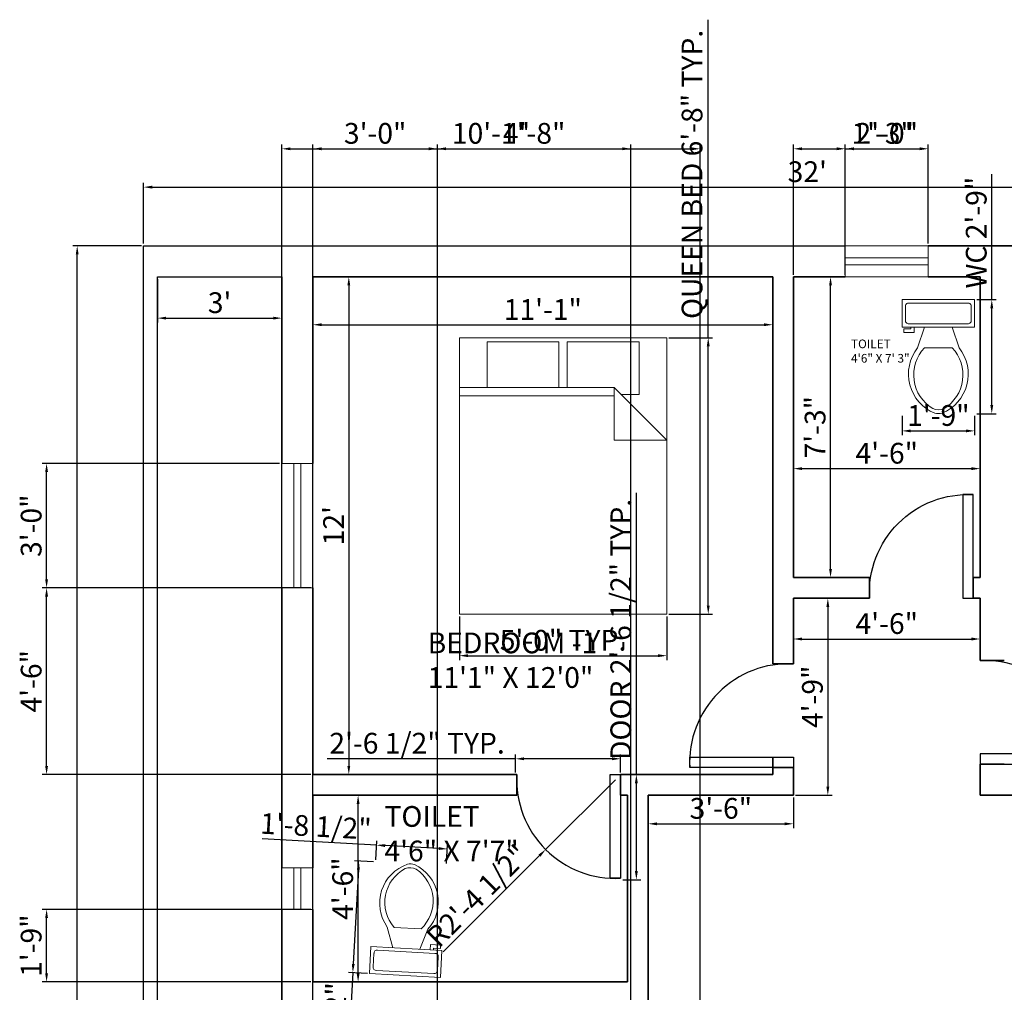
# Model space of a CAD drawing. Units: inches. Extents: x 2117 to 2588, y 1610 to 2201.
# Tile 3 of 4: x 2122 to 2407, y 1920 to 2201. Entities that reach past the tile are written whole.
import ezdxf

# ---------------------------------------------------------------- set-up
doc = ezdxf.new("R2010")
doc.units = ezdxf.units.IN
for name, color, linetype, lineweight in [('A-ANNO-DIMS', 2, 'Continuous', 18), ('A-AREA-IDEN', 7, 'Continuous', 25), ('A-DOOR', 4, 'Continuous', 25), ('A-FLOR-FIXT', 9, 'Continuous', 18), ('A-FURN', 8, 'Continuous', 18), ('A-WALL', 7, 'Continuous', 35), ('C-PROP', 7, 'Continuous', 30), ('WINDOW', 150, 'Continuous', 18)]:
    doc.layers.add(name, color=color, linetype=linetype, lineweight=lineweight)
doc.styles.get("Standard").update_dxf_attribs({"font": 'arial.ttf'})
doc.dimstyles.new('ISO-25', dxfattribs={"dimtxt": 6, "dimasz": 2.5, "dimexe": 1.25, "dimexo": 0.625, "dimtad": 1, "dimlunit": 3, "dimtxsty": 'Standard', "dimcen": 2.5, "dimadec": 0, "dimazin": 0, "dimtfac": 1, "dimtmove": 0, "dimatfit": 3, "dimfxl": 1, "dimarcsym": 0})

# ---------------------------------------------------------------- blocks, each defined once
blk = doc.blocks.new('*D3')
at = {"layer": 'A-ANNO-DIMS', "color": 0, "lineweight": -2, "transparency": 16777216}
for p, q in [((2346.08, 2126.4), (2346.08, 2070.29)), ((2400.08, 2126.4), (2400.08, 2070.29)), ((2348.58, 2071.54), (2397.58, 2071.54))]:
    blk.add_line(p, q, dxfattribs=at)
at = {"layer": 'A-ANNO-DIMS', "color": 0, "transparency": 16777216}
for points in [[(2348.58, 2071.95), (2348.58, 2071.12), (2346.08, 2071.54)], [(2397.58, 2071.95), (2397.58, 2071.12), (2400.08, 2071.54)]]:
    blk.add_solid(points, dxfattribs=at)
at = {"layer": 'Defpoints', "color": 0, "transparency": 16777216}
for p in [(2346.08, 2127.03), (2400.08, 2127.03), (2400.08, 2071.54)]:
    blk.add_point(p, dxfattribs=at)
at = {"layer": 'A-ANNO-DIMS', "color": 0, "transparency": 16777216, "insert": (2373.08, 2075.22), "char_height": 6, "attachment_point": 5}
blk.add_mtext('4\'-6"', dxfattribs=at)
blk = doc.blocks.new('*D4')
at = {"layer": 'A-ANNO-DIMS', "color": 0, "lineweight": -2, "transparency": 16777216}
for p, q in [((2207.7, 2127.03), (2218.7, 2127.03)), ((2217.45, 2124.53), (2217.45, 1985.53)), ((2207.7, 1983.03), (2218.7, 1983.03))]:
    blk.add_line(p, q, dxfattribs=at)
at = {"layer": 'A-ANNO-DIMS', "color": 0, "transparency": 16777216}
for points in [[(2217.04, 2124.53), (2217.87, 2124.53), (2217.45, 2127.03)], [(2217.04, 1985.53), (2217.87, 1985.53), (2217.45, 1983.03)]]:
    blk.add_solid(points, dxfattribs=at)
at = {"layer": 'Defpoints', "color": 0, "transparency": 16777216}
for p in [(2207.08, 2127.03), (2207.08, 1983.03), (2217.45, 1983.03)]:
    blk.add_point(p, dxfattribs=at)
at = {"layer": 'A-ANNO-DIMS', "color": 0, "transparency": 16777216, "insert": (2213.82, 2055.03), "char_height": 6, "attachment_point": 5, "rotation": 90}
blk.add_mtext("12'", dxfattribs=at)
blk = doc.blocks.new('*D7')
at = {"layer": 'A-ANNO-DIMS', "color": 0, "lineweight": -2, "transparency": 16777216}
for p, q in [((2207.7, 1977.03), (2221.4, 1977.03)), ((2220.15, 1925.53), (2220.15, 1974.53)), ((2207.7, 1923.03), (2221.4, 1923.03))]:
    blk.add_line(p, q, dxfattribs=at)
at = {"layer": 'A-ANNO-DIMS', "color": 0, "transparency": 16777216}
for points in [[(2219.73, 1974.53), (2220.56, 1974.53), (2220.15, 1977.03)], [(2219.73, 1925.53), (2220.56, 1925.53), (2220.15, 1923.03)]]:
    blk.add_solid(points, dxfattribs=at)
at = {"layer": 'Defpoints', "color": 0, "transparency": 16777216}
for p in [(2207.08, 1977.03), (2220.15, 1977.03), (2207.08, 1923.03)]:
    blk.add_point(p, dxfattribs=at)
at = {"layer": 'A-ANNO-DIMS', "color": 0, "transparency": 16777216, "insert": (2216.46, 1950.03), "char_height": 6, "attachment_point": 5, "rotation": 90}
blk.add_mtext('4\'-6"', dxfattribs=at)
blk = doc.blocks.new('*D9')
at = {"layer": 'A-ANNO-DIMS', "color": 0, "lineweight": -2, "transparency": 16777216}
for p, q in [((2162.08, 2126.4), (2162.08, 2113.83)), ((2198.08, 2126.4), (2198.08, 2113.83)), ((2164.58, 2115.08), (2195.58, 2115.08))]:
    blk.add_line(p, q, dxfattribs=at)
at = {"layer": 'A-ANNO-DIMS', "color": 0, "transparency": 16777216}
for points in [[(2164.58, 2115.5), (2164.58, 2114.67), (2162.08, 2115.08)], [(2195.58, 2115.5), (2195.58, 2114.67), (2198.08, 2115.08)]]:
    blk.add_solid(points, dxfattribs=at)
at = {"layer": 'Defpoints', "color": 0, "transparency": 16777216}
for p in [(2162.08, 2127.03), (2198.08, 2127.03), (2198.08, 2115.08)]:
    blk.add_point(p, dxfattribs=at)
at = {"layer": 'A-ANNO-DIMS', "color": 0, "transparency": 16777216, "insert": (2180.08, 2118.78), "char_height": 6, "attachment_point": 5}
blk.add_mtext("3'", dxfattribs=at)
blk = doc.blocks.new('*D10')
at = {"layer": 'A-ANNO-DIMS', "color": 0, "lineweight": -2, "transparency": 16777216}
for p, q in [((2207.08, 2126.4), (2207.08, 2111.92)), ((2340.08, 2126.4), (2340.08, 2111.92)), ((2209.58, 2113.17), (2337.58, 2113.17))]:
    blk.add_line(p, q, dxfattribs=at)
at = {"layer": 'A-ANNO-DIMS', "color": 0, "transparency": 16777216}
for points in [[(2209.58, 2113.59), (2209.58, 2112.76), (2207.08, 2113.17)], [(2337.58, 2113.59), (2337.58, 2112.76), (2340.08, 2113.17)]]:
    blk.add_solid(points, dxfattribs=at)
at = {"layer": 'Defpoints', "color": 0, "transparency": 16777216}
for p in [(2207.08, 2127.03), (2340.08, 2127.03), (2340.08, 2113.17)]:
    blk.add_point(p, dxfattribs=at)
at = {"layer": 'A-ANNO-DIMS', "color": 0, "transparency": 16777216, "insert": (2273.58, 2116.81), "char_height": 6, "attachment_point": 5}
blk.add_mtext('11\'-1"', dxfattribs=at)
blk = doc.blocks.new('*D11')
at = {"layer": 'A-ANNO-DIMS', "color": 0, "lineweight": -2, "transparency": 16777216}
for p, q in [((2346.7, 2127.03), (2358.06, 2127.03)), ((2356.81, 2042.53), (2356.81, 2124.53)), ((2346.7, 2040.03), (2358.06, 2040.03))]:
    blk.add_line(p, q, dxfattribs=at)
at = {"layer": 'A-ANNO-DIMS', "color": 0, "transparency": 16777216}
for points in [[(2356.39, 2124.53), (2357.22, 2124.53), (2356.81, 2127.03)], [(2356.39, 2042.53), (2357.22, 2042.53), (2356.81, 2040.03)]]:
    blk.add_solid(points, dxfattribs=at)
at = {"layer": 'Defpoints', "color": 0, "transparency": 16777216}
for p in [(2346.08, 2127.03), (2356.81, 2127.03), (2346.08, 2040.03)]:
    blk.add_point(p, dxfattribs=at)
at = {"layer": 'A-ANNO-DIMS', "color": 0, "transparency": 16777216, "insert": (2353.12, 2083.53), "char_height": 6, "attachment_point": 5, "rotation": 90}
blk.add_mtext('7\'-3"', dxfattribs=at)
blk = doc.blocks.new('*D12')
at = {"layer": 'A-ANNO-DIMS', "color": 0, "lineweight": -2, "transparency": 16777216}
for p, q in [((2346.7, 2034.03), (2357.28, 2034.03)), ((2356.03, 2031.53), (2356.03, 1979.53)), ((2346.7, 1977.03), (2357.28, 1977.03))]:
    blk.add_line(p, q, dxfattribs=at)
at = {"layer": 'A-ANNO-DIMS', "color": 0, "transparency": 16777216}
for points in [[(2355.61, 2031.53), (2356.44, 2031.53), (2356.03, 2034.03)], [(2355.61, 1979.53), (2356.44, 1979.53), (2356.03, 1977.03)]]:
    blk.add_solid(points, dxfattribs=at)
at = {"layer": 'Defpoints', "color": 0, "transparency": 16777216}
for p in [(2346.08, 2034.03), (2346.08, 1977.03), (2356.03, 1977.03)]:
    blk.add_point(p, dxfattribs=at)
at = {"layer": 'A-ANNO-DIMS', "color": 0, "transparency": 16777216, "insert": (2352.34, 2005.53), "char_height": 6, "attachment_point": 5, "rotation": 90}
blk.add_mtext('4\'-9"', dxfattribs=at)
blk = doc.blocks.new('*D13')
at = {"layer": 'A-ANNO-DIMS', "color": 0, "lineweight": -2, "transparency": 16777216}
for p, q in [((2346.08, 2033.4), (2346.08, 2021)), ((2400.08, 2033.4), (2400.08, 2021)), ((2348.58, 2022.25), (2397.58, 2022.25))]:
    blk.add_line(p, q, dxfattribs=at)
at = {"layer": 'A-ANNO-DIMS', "color": 0, "transparency": 16777216}
for points in [[(2348.58, 2022.67), (2348.58, 2021.83), (2346.08, 2022.25)], [(2397.58, 2022.67), (2397.58, 2021.83), (2400.08, 2022.25)]]:
    blk.add_solid(points, dxfattribs=at)
at = {"layer": 'Defpoints', "color": 0, "transparency": 16777216}
for p in [(2346.08, 2034.03), (2400.08, 2034.03), (2400.08, 2022.25)]:
    blk.add_point(p, dxfattribs=at)
at = {"layer": 'A-ANNO-DIMS', "color": 0, "transparency": 16777216, "insert": (2373.08, 2025.94), "char_height": 6, "attachment_point": 5}
blk.add_mtext('4\'-6"', dxfattribs=at)
blk = doc.blocks.new('*D14')
at = {"layer": 'A-ANNO-DIMS', "color": 0, "lineweight": -2, "transparency": 16777216}
for p, q in [((2304.08, 1976.4), (2304.08, 1967.53)), ((2346.08, 1976.4), (2346.08, 1967.53)), ((2306.58, 1968.78), (2343.58, 1968.78))]:
    blk.add_line(p, q, dxfattribs=at)
at = {"layer": 'A-ANNO-DIMS', "color": 0, "transparency": 16777216}
for points in [[(2306.58, 1969.19), (2306.58, 1968.36), (2304.08, 1968.78)], [(2343.58, 1969.19), (2343.58, 1968.36), (2346.08, 1968.78)]]:
    blk.add_solid(points, dxfattribs=at)
at = {"layer": 'Defpoints', "color": 0, "transparency": 16777216}
for p in [(2304.08, 1977.03), (2346.08, 1977.03), (2346.08, 1968.78)]:
    blk.add_point(p, dxfattribs=at)
at = {"layer": 'A-ANNO-DIMS', "color": 0, "transparency": 16777216, "insert": (2325.08, 1972.47), "char_height": 6, "attachment_point": 5}
blk.add_mtext('3\'-6"', dxfattribs=at)
blk = doc.blocks.new('Bed - Queen')
for p, q in [((0, -80.00003), (0, 0)), ((0, 0), (59.99999, 0)), ((59.99999, 0), (59.99999, -80.00003)), ((7.99999, -1.2), (28.79998, -1.2)), ((7.99999, -14.4), (7.99999, -1.2)), ((28.79998, -1.2), (28.79998, -14.4)), ((31.19999, -1.2), (51.99999, -1.2)), ((31.19999, -14.4), (31.19999, -1.2)), ((51.99999, -1.2), (51.99999, -16.4)), ((0, -14.4), (44.8, -14.4)), ((44.8, -16.8), (0, -16.8)), ((59.99999, -29.6), (44.8, -14.4)), ((44.8, -14.4), (44.8, -29.6)), ((51.99999, -16.4), (46.79936, -16.4)), ((44.8, -29.6), (59.99999, -29.6)), ((59.99999, -80.00003), (0, -80.00003))]:
    blk.add_line(p, q)
blk = doc.blocks.new('Toilet - top')
for p, q in [((9.5, -6), (9.5, -2)), ((-10, -8.5), (-8, -8.5)), ((-10, -9.5), (-10, -8.5)), ((-8, -8.5), (-8, -8)), ((-7, -8), (-7, -9.5)), ((-4, -8), (-6, -14)), ((4, -8), (6, -14)), ((-7, -9.5), (-10, -9.5)), ((4, -14), (-4, -14))]:
    blk.add_line(p, q)
blk.add_lwpolyline([(10.5, -8), (10.5, 0), (-10.5, 0), (-10.5, -8)], close=True)
for points in [[(-9.5, -2), (-9.5, -6)], [(8.5, -1), (-8.5, -1)], [(-8.5, -7), (8.5, -7)]]:
    blk.add_lwpolyline(points)
for centre, radius, start, end in [((-8.62, -1.88), 0.884, 81.8699, 188.1301), ((8.62, -1.88), 0.884, 351.8699, 98.1301), ((-8.62, -6.12), 0.884, 171.8699, 278.1301), ((8.62, -6.12), 0.884, 261.8699, 8.1301), ((3.52, -21.58), 12.17, 141.4691, 247.9714), ((4.2, -21.82), 11.33, 136.3677, 238.9468), ((-3.52, -21.58), 12.17, 292.0284, 38.5307), ((-4.2, -21.82), 11.33, 301.053, 43.6321), ((0, -27.88), 4, 245.7318, 294.2682), ((0, -29), 4, 254.8605, 285.1395)]:
    blk.add_arc(centre, radius, start, end)
blk = doc.blocks.new('*D30')
at = {"layer": 'A-ANNO-DIMS', "color": 0, "lineweight": -2, "transparency": 16777216}
for p, q in [((2158.08, 2136.65), (2158.08, 2154.24)), ((2542.08, 2136.65), (2542.08, 2154.24)), ((2160.58, 2152.99), (2539.58, 2152.99))]:
    blk.add_line(p, q, dxfattribs=at)
at = {"layer": 'A-ANNO-DIMS', "color": 0, "transparency": 16777216}
for points in [[(2160.58, 2153.4), (2160.58, 2152.57), (2158.08, 2152.99)], [(2539.58, 2153.4), (2539.58, 2152.57), (2542.08, 2152.99)]]:
    blk.add_solid(points, dxfattribs=at)
at = {"layer": 'Defpoints', "color": 0, "transparency": 16777216}
for p in [(2542.08, 2152.99), (2158.08, 2136.03), (2542.08, 2136.03)]:
    blk.add_point(p, dxfattribs=at)
at = {"layer": 'A-ANNO-DIMS', "color": 0, "transparency": 16777216, "insert": (2350.08, 2156.68), "char_height": 6, "attachment_point": 5}
blk.add_mtext("32'", dxfattribs=at)
blk = doc.blocks.new('*D33')
at = {"layer": 'A-ANNO-DIMS', "color": 0, "lineweight": -2, "transparency": 16777216}
for p, q in [((2157.45, 2136.03), (2137.63, 2136.03)), ((2138.88, 1658.53), (2138.88, 2133.53)), ((2157.45, 1656.03), (2137.63, 1656.03))]:
    blk.add_line(p, q, dxfattribs=at)
at = {"layer": 'A-ANNO-DIMS', "color": 0, "transparency": 16777216}
for points in [[(2138.47, 2133.53), (2139.3, 2133.53), (2138.88, 2136.03)], [(2138.47, 1658.53), (2139.3, 1658.53), (2138.88, 1656.03)]]:
    blk.add_solid(points, dxfattribs=at)
at = {"layer": 'Defpoints', "color": 0, "transparency": 16777216}
for p in [(2138.88, 2136.03), (2158.08, 2136.03), (2158.08, 1656.03)]:
    blk.add_point(p, dxfattribs=at)
at = {"layer": 'A-ANNO-DIMS', "color": 0, "transparency": 16777216, "insert": (2135.2, 1896.03), "char_height": 6, "attachment_point": 5, "rotation": 90}
blk.add_mtext("40'", dxfattribs=at)
blk = doc.blocks.new('WIN-12IN-9IN-WALL')
for p, q in [((9, 12), (0, 12)), ((0, 0), (0, 12)), ((3.5, 0), (3.5, 12)), ((5.5, 0), (5.5, 12)), ((9, 0), (9, 12)), ((9, 0), (0, 0))]:
    blk.add_line(p, q)
blk = doc.blocks.new('DOOR-SWING-30IN')
blk.add_lwpolyline([(30.04, 0), (0.04, 0), (0.04, 3), (30.04, 3)], close=True)
blk.add_arc((28.54, 1.5), 28.54, 86.9872, 183.0128)
blk = doc.blocks.new('*D41')
at = {"layer": 'A-ANNO-DIMS', "color": 0, "lineweight": -2, "transparency": 16777216}
for p, q in [((2300.64, 1983.03), (2300.64, 2064.51)), ((2296.7, 1983.03), (2301.89, 1983.03)), ((2300.64, 1955.1), (2300.64, 1980.53)), ((2296.7, 1952.6), (2301.89, 1952.6))]:
    blk.add_line(p, q, dxfattribs=at)
at = {"layer": 'A-ANNO-DIMS', "color": 0, "transparency": 16777216}
for points in [[(2300.22, 1980.53), (2301.06, 1980.53), (2300.64, 1983.03)], [(2300.22, 1955.1), (2301.06, 1955.1), (2300.64, 1952.6)]]:
    blk.add_solid(points, dxfattribs=at)
at = {"layer": 'Defpoints', "color": 0, "transparency": 16777216}
for p in [(2296.08, 1983.03), (2300.64, 1983.03), (2296.08, 1952.6)]:
    blk.add_point(p, dxfattribs=at)
at = {"layer": 'A-ANNO-DIMS', "color": 0, "transparency": 16777216, "insert": (2296.91, 2025.02), "char_height": 6, "attachment_point": 5, "rotation": 90}
blk.add_mtext('DOOR 2\'-6 1/2" TYP.', dxfattribs=at)
blk = doc.blocks.new('*D42')
at = {"layer": 'A-ANNO-DIMS', "color": 0, "lineweight": -2, "transparency": 16777216}
for p, q in [((2265.65, 1983.65), (2265.65, 1988.84)), ((2296.08, 1983.65), (2296.08, 1988.84)), ((2265.65, 1987.59), (2211.24, 1987.59)), ((2293.58, 1987.59), (2268.15, 1987.59))]:
    blk.add_line(p, q, dxfattribs=at)
at = {"layer": 'A-ANNO-DIMS', "color": 0, "transparency": 16777216}
for points in [[(2268.15, 1988.01), (2268.15, 1987.18), (2265.65, 1987.59)], [(2293.58, 1988.01), (2293.58, 1987.18), (2296.08, 1987.59)]]:
    blk.add_solid(points, dxfattribs=at)
at = {"layer": 'Defpoints', "color": 0, "transparency": 16777216}
for p in [(2265.65, 1987.59), (2265.65, 1983.03), (2296.08, 1983.03)]:
    blk.add_point(p, dxfattribs=at)
at = {"layer": 'A-ANNO-DIMS', "color": 0, "transparency": 16777216, "insert": (2237.2, 1991.32), "char_height": 6, "attachment_point": 5}
blk.add_mtext('2\'-6 1/2" TYP.', dxfattribs=at)
blk = doc.blocks.new('*D43')
at = {"layer": 'A-ANNO-DIMS', "color": 0, "lineweight": -2, "transparency": 16777216}
for p, q in [((2321.43, 2109.42), (2321.43, 2201.43)), ((2310.06, 2109.42), (2322.68, 2109.42)), ((2321.43, 2031.92), (2321.43, 2106.92)), ((2310.06, 2029.42), (2322.68, 2029.42))]:
    blk.add_line(p, q, dxfattribs=at)
at = {"layer": 'A-ANNO-DIMS', "color": 0, "transparency": 16777216}
for points in [[(2321.01, 2106.92), (2321.85, 2106.92), (2321.43, 2109.42)], [(2321.01, 2031.92), (2321.85, 2031.92), (2321.43, 2029.42)]]:
    blk.add_solid(points, dxfattribs=at)
at = {"layer": 'Defpoints', "color": 0, "transparency": 16777216}
for p in [(2309.43, 2109.42), (2321.43, 2109.42), (2309.43, 2029.42)]:
    blk.add_point(p, dxfattribs=at)
at = {"layer": 'A-ANNO-DIMS', "color": 0, "transparency": 16777216, "insert": (2317.52, 2156.68), "char_height": 6, "attachment_point": 5, "rotation": 90}
blk.add_mtext('QUEEN BED 6\'-8" TYP.', dxfattribs=at)
blk = doc.blocks.new('*D44')
at = {"layer": 'A-ANNO-DIMS', "color": 0, "lineweight": -2, "transparency": 16777216}
for p, q in [((2249.43, 2028.8), (2249.43, 2016.17)), ((2309.43, 2028.8), (2309.43, 2016.17)), ((2251.93, 2017.42), (2306.93, 2017.42))]:
    blk.add_line(p, q, dxfattribs=at)
at = {"layer": 'A-ANNO-DIMS', "color": 0, "transparency": 16777216}
for points in [[(2251.93, 2017.84), (2251.93, 2017.01), (2249.43, 2017.42)], [(2306.93, 2017.84), (2306.93, 2017.01), (2309.43, 2017.42)]]:
    blk.add_solid(points, dxfattribs=at)
at = {"layer": 'Defpoints', "color": 0, "transparency": 16777216}
for p in [(2249.43, 2029.42), (2309.43, 2029.42), (2309.43, 2017.42)]:
    blk.add_point(p, dxfattribs=at)
at = {"layer": 'A-ANNO-DIMS', "color": 0, "transparency": 16777216, "insert": (2279.43, 2021.11), "char_height": 6, "attachment_point": 5}
blk.add_mtext('5\'-0" TYP.', dxfattribs=at)
blk = doc.blocks.new('*D45')
at = {"layer": 'A-ANNO-DIMS', "color": 0, "lineweight": -2, "transparency": 16777216}
for p, q in [((2224.57, 1957.8), (2219.1, 1958.1)), ((2220.21, 1955.54), (2218.73, 1928.23)), ((2218.6, 1925.73), (2215.87, 1875.58)), ((2222.82, 1925.5), (2217.35, 1925.8))]:
    blk.add_line(p, q, dxfattribs=at)
at = {"layer": 'A-ANNO-DIMS', "color": 0, "transparency": 16777216}
for points in [[(2219.8, 1955.56), (2220.63, 1955.51), (2220.35, 1958.03)], [(2218.32, 1928.25), (2219.15, 1928.2), (2218.6, 1925.73)]]:
    blk.add_solid(points, dxfattribs=at)
at = {"layer": 'Defpoints', "color": 0, "transparency": 16777216}
for p in [(2225.19, 1957.77), (2218.6, 1925.73), (2223.44, 1925.47)]:
    blk.add_point(p, dxfattribs=at)
at = {"layer": 'A-ANNO-DIMS', "color": 0, "transparency": 16777216, "insert": (2213.45, 1899.61), "char_height": 6, "attachment_point": 5, "rotation": 86.894}
blk.add_mtext('WC 2\'-8 1/2"', dxfattribs=at)
blk = doc.blocks.new('*D46')
at = {"layer": 'A-ANNO-DIMS', "color": 0, "lineweight": -2, "transparency": 16777216}
for p, q in [((2225.46, 1962.61), (2192.39, 1964.41)), ((2225.23, 1958.39), (2225.52, 1963.86)), ((2243.49, 1961.64), (2227.95, 1962.48)), ((2245.76, 1957.28), (2246.05, 1962.75))]:
    blk.add_line(p, q, dxfattribs=at)
at = {"layer": 'A-ANNO-DIMS', "color": 0, "transparency": 16777216}
for points in [[(2227.98, 1962.9), (2227.93, 1962.06), (2225.46, 1962.61)], [(2243.51, 1962.05), (2243.47, 1961.22), (2245.98, 1961.5)]]:
    blk.add_solid(points, dxfattribs=at)
at = {"layer": 'Defpoints', "color": 0, "transparency": 16777216}
for p in [(2225.46, 1962.61), (2225.19, 1957.77), (2245.72, 1956.66)]:
    blk.add_point(p, dxfattribs=at)
at = {"layer": 'A-ANNO-DIMS', "color": 0, "transparency": 16777216, "insert": (2207.88, 1967.3), "char_height": 6, "attachment_point": 5, "rotation": 356.894}
blk.add_mtext('1\'-8 1/2"', dxfattribs=at)
blk = doc.blocks.new('*D47')
at = {"layer": 'A-ANNO-DIMS', "color": 0, "lineweight": -2, "transparency": 16777216}
for p, q in [((2403.45, 2120.46), (2403.45, 2156.7)), ((2399.12, 2120.46), (2404.7, 2120.46)), ((2403.45, 2089.91), (2403.45, 2117.96)), ((2399.12, 2087.41), (2404.7, 2087.41))]:
    blk.add_line(p, q, dxfattribs=at)
at = {"layer": 'A-ANNO-DIMS', "color": 0, "transparency": 16777216}
for points in [[(2403.04, 2117.96), (2403.87, 2117.96), (2403.45, 2120.46)], [(2403.04, 2089.91), (2403.87, 2089.91), (2403.45, 2087.41)]]:
    blk.add_solid(points, dxfattribs=at)
at = {"layer": 'Defpoints', "color": 0, "transparency": 16777216}
for p in [(2398.5, 2120.46), (2403.45, 2120.46), (2398.5, 2087.41)]:
    blk.add_point(p, dxfattribs=at)
at = {"layer": 'A-ANNO-DIMS', "color": 0, "transparency": 16777216, "insert": (2399.73, 2139.83), "char_height": 6, "attachment_point": 5, "rotation": 90}
blk.add_mtext('WC 2\'-9"', dxfattribs=at)
blk = doc.blocks.new('*D48')
at = {"layer": 'A-ANNO-DIMS', "color": 0, "lineweight": -2, "transparency": 16777216}
for p, q in [((2377.5, 2086.79), (2377.5, 2081.21)), ((2398.5, 2086.79), (2398.5, 2081.21)), ((2380, 2082.46), (2396, 2082.46))]:
    blk.add_line(p, q, dxfattribs=at)
at = {"layer": 'A-ANNO-DIMS', "color": 0, "transparency": 16777216}
for points in [[(2380, 2082.87), (2380, 2082.04), (2377.5, 2082.46)], [(2396, 2082.87), (2396, 2082.04), (2398.5, 2082.46)]]:
    blk.add_solid(points, dxfattribs=at)
at = {"layer": 'Defpoints', "color": 0, "transparency": 16777216}
for p in [(2377.5, 2087.41), (2398.5, 2087.41), (2398.5, 2082.46)]:
    blk.add_point(p, dxfattribs=at)
at = {"layer": 'A-ANNO-DIMS', "color": 0, "transparency": 16777216, "insert": (2388, 2086.14), "char_height": 6, "attachment_point": 5}
blk.add_mtext('1\'-9"', dxfattribs=at)
blk = doc.blocks.new('*D58')
at = {"layer": 'A-ANNO-DIMS', "color": 0, "lineweight": -2, "transparency": 16777216}
for p, q in [((2198.08, 1696.65), (2198.08, 2165.33)), ((2319.08, 1696.65), (2319.08, 2165.33)), ((2200.58, 2164.08), (2316.58, 2164.08))]:
    blk.add_line(p, q, dxfattribs=at)
at = {"layer": 'A-ANNO-DIMS', "color": 0, "transparency": 16777216}
for points in [[(2200.58, 2164.5), (2200.58, 2163.66), (2198.08, 2164.08)], [(2316.58, 2164.5), (2316.58, 2163.66), (2319.08, 2164.08)]]:
    blk.add_solid(points, dxfattribs=at)
at = {"layer": 'Defpoints', "color": 0, "transparency": 16777216}
for p in [(2319.08, 2164.08), (2198.08, 1696.03), (2319.08, 1696.03)]:
    blk.add_point(p, dxfattribs=at)
at = {"layer": 'A-ANNO-DIMS', "color": 0, "transparency": 16777216, "insert": (2258.58, 2167.77), "char_height": 6, "attachment_point": 5}
blk.add_mtext('10\'-1"', dxfattribs=at)
blk = doc.blocks.new('*D60')
at = {"layer": 'A-ANNO-DIMS', "color": 0, "lineweight": -2, "transparency": 16777216}
for p, q in [((2243.08, 1832.65), (2243.08, 2165.33)), ((2299.08, 1832.65), (2299.08, 2165.33)), ((2245.58, 2164.08), (2296.58, 2164.08))]:
    blk.add_line(p, q, dxfattribs=at)
at = {"layer": 'A-ANNO-DIMS', "color": 0, "transparency": 16777216}
for points in [[(2245.58, 2164.5), (2245.58, 2163.66), (2243.08, 2164.08)], [(2296.58, 2164.5), (2296.58, 2163.66), (2299.08, 2164.08)]]:
    blk.add_solid(points, dxfattribs=at)
at = {"layer": 'Defpoints', "color": 0, "transparency": 16777216}
for p in [(2299.08, 2164.08), (2243.08, 1832.03), (2299.08, 1832.03)]:
    blk.add_point(p, dxfattribs=at)
at = {"layer": 'A-ANNO-DIMS', "color": 0, "transparency": 16777216, "insert": (2271.08, 2167.77), "char_height": 6, "attachment_point": 5}
blk.add_mtext('4\'-8"', dxfattribs=at)
blk = doc.blocks.new('*D61')
at = {"layer": 'A-ANNO-DIMS', "color": 0, "lineweight": -2, "transparency": 16777216}
for p, q in [((2197.45, 2073.03), (2128.78, 2073.03)), ((2130.03, 2039.53), (2130.03, 2070.53)), ((2197.45, 2037.03), (2128.78, 2037.03))]:
    blk.add_line(p, q, dxfattribs=at)
at = {"layer": 'A-ANNO-DIMS', "color": 0, "transparency": 16777216}
for points in [[(2129.61, 2070.53), (2130.44, 2070.53), (2130.03, 2073.03)], [(2129.61, 2039.53), (2130.44, 2039.53), (2130.03, 2037.03)]]:
    blk.add_solid(points, dxfattribs=at)
at = {"layer": 'Defpoints', "color": 0, "transparency": 16777216}
for p in [(2130.03, 2073.03), (2198.08, 2073.03), (2198.08, 2037.03)]:
    blk.add_point(p, dxfattribs=at)
at = {"layer": 'A-ANNO-DIMS', "color": 0, "transparency": 16777216, "insert": (2126.34, 2055.03), "char_height": 6, "attachment_point": 5, "rotation": 90}
blk.add_mtext('3\'-0"', dxfattribs=at)
blk = doc.blocks.new('*D62')
at = {"layer": 'A-ANNO-DIMS', "color": 0, "lineweight": -2, "transparency": 16777216}
for p, q in [((2206.45, 2037.03), (2128.78, 2037.03)), ((2130.03, 1985.53), (2130.03, 2034.53)), ((2206.45, 1983.03), (2128.78, 1983.03))]:
    blk.add_line(p, q, dxfattribs=at)
at = {"layer": 'A-ANNO-DIMS', "color": 0, "transparency": 16777216}
for points in [[(2129.61, 2034.53), (2130.44, 2034.53), (2130.03, 2037.03)], [(2129.61, 1985.53), (2130.44, 1985.53), (2130.03, 1983.03)]]:
    blk.add_solid(points, dxfattribs=at)
at = {"layer": 'Defpoints', "color": 0, "transparency": 16777216}
for p in [(2130.03, 2037.03), (2207.08, 2037.03), (2207.08, 1983.03)]:
    blk.add_point(p, dxfattribs=at)
at = {"layer": 'A-ANNO-DIMS', "color": 0, "transparency": 16777216, "insert": (2126.34, 2010.03), "char_height": 6, "attachment_point": 5, "rotation": 90}
blk.add_mtext('4\'-6"', dxfattribs=at)
blk = doc.blocks.new('*D63')
at = {"layer": 'A-ANNO-DIMS', "color": 0, "lineweight": -2, "transparency": 16777216}
for p, q in [((2361.08, 2136.65), (2361.08, 2165.33)), ((2385.08, 2136.65), (2385.08, 2165.33)), ((2363.58, 2164.08), (2382.58, 2164.08))]:
    blk.add_line(p, q, dxfattribs=at)
at = {"layer": 'A-ANNO-DIMS', "color": 0, "transparency": 16777216}
for points in [[(2363.58, 2164.5), (2363.58, 2163.66), (2361.08, 2164.08)], [(2382.58, 2164.5), (2382.58, 2163.66), (2385.08, 2164.08)]]:
    blk.add_solid(points, dxfattribs=at)
at = {"layer": 'Defpoints', "color": 0, "transparency": 16777216}
for p in [(2385.08, 2164.08), (2361.08, 2136.03), (2385.08, 2136.03)]:
    blk.add_point(p, dxfattribs=at)
at = {"layer": 'A-ANNO-DIMS', "color": 0, "transparency": 16777216, "insert": (2373.08, 2167.77), "char_height": 6, "attachment_point": 5}
blk.add_mtext('2\'-0"', dxfattribs=at)
blk = doc.blocks.new('*D64')
at = {"layer": 'A-ANNO-DIMS', "color": 0, "lineweight": -2, "transparency": 16777216}
for p, q in [((2346.08, 2127.65), (2346.08, 2165.33)), ((2361.08, 2127.65), (2361.08, 2165.33)), ((2348.58, 2164.08), (2358.58, 2164.08)), ((2361.08, 2164.08), (2380.21, 2164.08))]:
    blk.add_line(p, q, dxfattribs=at)
at = {"layer": 'A-ANNO-DIMS', "color": 0, "transparency": 16777216}
for points in [[(2348.58, 2164.5), (2348.58, 2163.66), (2346.08, 2164.08)], [(2358.58, 2164.5), (2358.58, 2163.66), (2361.08, 2164.08)]]:
    blk.add_solid(points, dxfattribs=at)
at = {"layer": 'Defpoints', "color": 0, "transparency": 16777216}
for p in [(2361.08, 2164.08), (2346.08, 2127.03), (2361.08, 2127.03)]:
    blk.add_point(p, dxfattribs=at)
at = {"layer": 'A-ANNO-DIMS', "color": 0, "transparency": 16777216, "insert": (2371.89, 2167.77), "char_height": 6, "attachment_point": 5}
blk.add_mtext('1\'-3"', dxfattribs=at)
blk = doc.blocks.new('*D71')
at = {"layer": 'A-ANNO-DIMS', "color": 0, "lineweight": -2, "transparency": 16777216}
for p, q in [((2206.45, 1944.03), (2128.78, 1944.03)), ((2130.03, 1925.53), (2130.03, 1941.53)), ((2206.45, 1923.03), (2128.78, 1923.03))]:
    blk.add_line(p, q, dxfattribs=at)
at = {"layer": 'A-ANNO-DIMS', "color": 0, "transparency": 16777216}
for points in [[(2129.61, 1941.53), (2130.44, 1941.53), (2130.03, 1944.03)], [(2129.61, 1925.53), (2130.44, 1925.53), (2130.03, 1923.03)]]:
    blk.add_solid(points, dxfattribs=at)
at = {"layer": 'Defpoints', "color": 0, "transparency": 16777216}
for p in [(2130.03, 1944.03), (2207.08, 1944.03), (2207.08, 1923.03)]:
    blk.add_point(p, dxfattribs=at)
at = {"layer": 'A-ANNO-DIMS', "color": 0, "transparency": 16777216, "insert": (2126.34, 1933.53), "char_height": 6, "attachment_point": 5, "rotation": 90}
blk.add_mtext('1\'-9"', dxfattribs=at)
blk = doc.blocks.new('*D76')
at = {"layer": 'A-ANNO-DIMS', "color": 0, "lineweight": -2, "transparency": 16777216}
for p, q in [((2207.08, 1832.65), (2207.08, 2165.33)), ((2243.08, 1832.65), (2243.08, 2165.33)), ((2209.58, 2164.08), (2240.58, 2164.08))]:
    blk.add_line(p, q, dxfattribs=at)
at = {"layer": 'A-ANNO-DIMS', "color": 0, "transparency": 16777216}
for points in [[(2209.58, 2164.5), (2209.58, 2163.66), (2207.08, 2164.08)], [(2240.58, 2164.5), (2240.58, 2163.66), (2243.08, 2164.08)]]:
    blk.add_solid(points, dxfattribs=at)
at = {"layer": 'Defpoints', "color": 0, "transparency": 16777216}
for p in [(2243.08, 2164.08), (2207.08, 1832.03), (2243.08, 1832.03)]:
    blk.add_point(p, dxfattribs=at)
at = {"layer": 'A-ANNO-DIMS', "color": 0, "transparency": 16777216, "insert": (2225.08, 2167.77), "char_height": 6, "attachment_point": 5}
blk.add_mtext('3\'-0"', dxfattribs=at)
blk = doc.blocks.new('*D78')
at = {"layer": 'A-ANNO-DIMS', "color": 0, "lineweight": -2, "transparency": 16777216}
for p, q in [((2294.58, 1981.53), (2274.4, 1961.35)), ((2244.75, 1931.7), (2272.63, 1959.58))]:
    blk.add_line(p, q, dxfattribs=at)
at = {"layer": 'A-ANNO-DIMS', "color": 0, "transparency": 16777216}
blk.add_solid([(2272.33, 1959.88), (2272.92, 1959.29), (2274.4, 1961.35)], dxfattribs=at)
at = {"layer": 'Defpoints', "color": 0, "transparency": 16777216}
for p in [(2294.58, 1981.53), (2274.4, 1961.35)]:
    blk.add_point(p, dxfattribs=at)
at = {"layer": 'A-ANNO-DIMS', "color": 0, "transparency": 16777216, "insert": (2255.17, 1947.39), "char_height": 6, "attachment_point": 5, "rotation": 44.9995}
blk.add_mtext('R2\'-4 1/2"', dxfattribs=at)

msp = doc.modelspace()

# ---------------------------------------------------------------- linework, layer by layer
at = {"layer": 'A-WALL'}
for p, q in [((2198.076, 2073.029), (2198.076, 2127.029)), ((2207.076, 2127.029), (2340.076, 2127.029)), ((2207.076, 2073.029), (2207.076, 2127.029)), ((2340.076, 2015.029), (2340.076, 2127.029)), ((2346.076, 2127.029), (2361.076, 2127.029)), ((2346.076, 2040.029), (2346.076, 2127.029)), ((2385.076, 2127.029), (2400.076, 2127.029)), ((2400.076, 2040.029), (2400.076, 2127.029)), ((2346.076, 2040.029), (2368.076, 2040.029)), ((2368.076, 2040.029), (2368.076, 2034.029)), ((2398.076, 2040.029), (2398.076, 2034.029)), ((2398.076, 2040.029), (2400.076, 2040.029)), ((2198.076, 1956.029), (2198.076, 2037.029)), ((2207.076, 1983.029), (2207.076, 2037.029)), ((2346.076, 2034.029), (2368.076, 2034.029)), ((2346.076, 2015.029), (2346.076, 2034.029)), ((2398.076, 2034.029), (2400.076, 2034.029)), ((2400.076, 2016.029), (2400.076, 2034.029)), ((2340.076, 2015.029), (2346.076, 2015.029)), ((2407.076, 2016.029), (2400.076, 2016.029)), ((2340.076, 1983.029), (2340.076, 1988.029)), ((2400.076, 1977.029), (2400.076, 1986.029)), ((2407.076, 1986.029), (2400.076, 1986.029)), ((2207.076, 1983.029), (2266.076, 1983.029)), ((2266.076, 1977.029), (2266.076, 1983.029)), ((2296.076, 1977.029), (2296.076, 1983.029)), ((2296.076, 1983.029), (2340.076, 1983.029)), ((2340.076, 1985.029), (2346.076, 1985.029)), ((2346.076, 1977.029), (2346.076, 1985.029)), ((2207.076, 1977.029), (2266.076, 1977.029)), ((2207.076, 1956.029), (2207.076, 1977.029)), ((2296.076, 1977.029), (2298.076, 1977.029)), ((2298.076, 1923.029), (2298.076, 1977.029)), ((2304.076, 1917.029), (2304.076, 1977.029)), ((2304.076, 1977.029), (2346.076, 1977.029)), ((2400.076, 1977.029), (2533.076, 1977.029)), ((2198.076, 1901.529), (2198.076, 1944.029)), ((2207.076, 1923.029), (2207.076, 1944.029)), ((2207.076, 1923.029), (2298.076, 1923.029))]:
    msp.add_line(p, q, dxfattribs=at)
msp.add_lwpolyline([(2385.076, 2136.029), (2542.076, 2136.029), (2542.076, 2079.029)], dxfattribs=at)
at = {"layer": 'C-PROP'}
for p, q in [((2162.076, 1660.029), (2162.076, 2127.029)), ((2162.076, 2127.029), (2198.076, 2127.029))]:
    msp.add_line(p, q, dxfattribs=at)
msp.add_lwpolyline([(2350.076, 1656.029), (2158.076, 1656.029), (2158.076, 2136.029), (2361.076, 2136.029)], dxfattribs=at)
at = {"layer": 'WINDOW'}
for p, q in [((2361.076, 2127.029), (2361.076, 2136.029)), ((2361.076, 2136.029), (2385.076, 2136.029)), ((2385.076, 2127.029), (2385.076, 2136.029)), ((2385.076, 2132.529), (2361.076, 2132.529)), ((2385.076, 2130.529), (2361.076, 2130.529)), ((2361.076, 2127.029), (2385.076, 2127.029)), ((2207.076, 2073.029), (2198.076, 2073.029)), ((2198.076, 2037.029), (2198.076, 2073.029)), ((2201.576, 2037.029), (2201.576, 2073.029)), ((2203.576, 2037.029), (2203.576, 2073.029)), ((2207.076, 2037.029), (2207.076, 2073.029)), ((2207.076, 2037.029), (2198.076, 2037.029))]:
    msp.add_line(p, q, dxfattribs=at)

# ---------------------------------------------------------------- block references
at = {"layer": 'A-DOOR', "extrusion": (0, 0, -1), "zscale": -1, "rotation": 270.0000000000016}
msp.add_blockref('DOOR-SWING-30IN', (-2398.075, 2064.068), dxfattribs=at)
at = {"layer": 'A-DOOR'}
msp.add_blockref('DOOR-SWING-30IN', (2316.036, 1985.029), dxfattribs=at)
at = {"layer": 'A-DOOR', "extrusion": (0, 0, -1), "zscale": -1}
msp.add_blockref('DOOR-SWING-30IN', (-2430.116, 1986.029), dxfattribs=at)
at = {"layer": 'A-DOOR', "rotation": 90.00000000000043}
msp.add_blockref('DOOR-SWING-30IN', (2296.075, 1952.989), dxfattribs=at)
at = {"layer": 'A-FLOR-FIXT'}
msp.add_blockref('Toilet - top', (2387.997, 2120.458), dxfattribs=at)
at = {"layer": 'A-FLOR-FIXT', "xscale": 0.9789467869854404, "yscale": 0.9789467869854404, "zscale": 0.9789467869854404, "rotation": 176.8940410564793}
msp.add_blockref('Toilet - top', (2233.705, 1924.909), dxfattribs=at)
at = {"layer": 'A-FURN'}
msp.add_blockref('Bed - Queen', (2249.43, 2109.422), dxfattribs=at)
at = {"layer": 'WINDOW'}
msp.add_blockref('WIN-12IN-9IN-WALL', (2198.076, 1944.029), dxfattribs=at)

# ---------------------------------------------------------------- texts
at = {"layer": 'A-AREA-IDEN', "attachment_point": 1}
for s, width, insert, char_height in [('{\\fArial|b1|i0|c0|p34;TOILET \\P4\'6" X 7\' 3" }', 43.26833, (2362.735, 2108.891), 2.5), ('{\\fArial|b1|i0|c0|p34;BEDROOM -1 \\P11\'1" X 12\'0"}', 64.79151, (2240.269, 2024.119), 6), ('{\\fArial|b1|i0|c0|p34;TOILET \\P4\'6" X 7\'7"}', 40.82788, (2227.768, 1973.911), 6)]:
    msp.add_mtext_dynamic_manual_height_columns(s, width=width, gutter_width=12.5, heights=[0], dxfattribs=dict(at, insert=insert, char_height=char_height))

# ---------------------------------------------------------------- dimensions: what is measured, and where the dimension line sits
at = {"layer": 'A-ANNO-DIMS'}
for base, p1, p2, angle, text, picture, middle in [((2321.43, 2109.422), (2309.43, 2029.422), (2309.43, 2109.422), 90, 'QUEEN BED <> TYP.', '*D43', (2317.519, 2156.677)), ((2403.454, 2120.458), (2398.497, 2087.412), (2398.497, 2120.458), 90, 'WC <>', '*D47', (2399.726, 2139.827)), ((2300.64, 1983.029), (2296.076, 1952.603), (2296.076, 1983.029), 90, 'DOOR <> TYP.', '*D41', (2296.91, 2025.018)), ((2265.651, 1987.592), (2296.076, 1983.029), (2265.651, 1983.029), 180, '<> TYP.', '*D42', (2237.198, 1991.32)), ((2218.596, 1925.729), (2225.194, 1957.769), (2223.441, 1925.466), 266.89404, 'WC <>', '*D45', (2213.446, 1899.61))]:
    dim = msp.add_linear_dim(base=base, p1=p1, p2=p2, angle=angle, text=text, dimstyle='ISO-25', override={"dimdec": 1, "dimlfac": 1, "dimrnd": 0, "dimzin": 1, "dimdsep": 46, "dimlunit": 4, "dimfrac": 2}, dxfattribs=at)
    dim.commit()
    dim.dimension.update_dxf_attribs({"geometry": picture, "text_midpoint": middle})
for base, p1, p2, override, picture, middle in [((2319.076, 2164.079), (2198.076, 1696.029), (2319.076, 1696.029), {"dimdec": 1, "dimlfac": 1, "dimrnd": 0, "dimzin": 1, "dimdsep": 46, "dimlunit": 4, "dimfrac": 2}, '*D58', (2258.576, 2167.767)), ((2243.076, 2164.079), (2207.076, 1832.029), (2243.076, 1832.029), {"dimdec": 1, "dimlfac": 1, "dimrnd": 0, "dimzin": 1, "dimdsep": 46, "dimlunit": 4, "dimfrac": 2}, '*D76', (2225.076, 2167.769)), ((2299.076, 2164.079), (2243.076, 1832.029), (2299.076, 1832.029), {"dimdec": 1, "dimlfac": 1, "dimrnd": 0, "dimzin": 1, "dimdsep": 46, "dimlunit": 4, "dimfrac": 2}, '*D60', (2271.076, 2167.767)), ((2361.076, 2164.079), (2346.076, 2127.029), (2361.076, 2127.029), {"dimdec": 1, "dimlfac": 1, "dimrnd": 0, "dimzin": 1, "dimdsep": 46, "dimlunit": 4, "dimfrac": 2}, '*D64', (2371.893, 2167.769)), ((2385.076, 2164.079), (2361.076, 2136.029), (2385.076, 2136.029), {"dimdec": 1, "dimlfac": 1, "dimrnd": 0, "dimzin": 1, "dimdsep": 46, "dimlunit": 4, "dimfrac": 2}, '*D63', (2373.076, 2167.767)), ((2542.076, 2152.986), (2158.076, 2136.029), (2542.076, 2136.029), {"dimclrd": 0, "dimclre": 0, "dimclrt": 0}, '*D30', (2350.076, 2156.677)), ((2198.076, 2115.085), (2162.076, 2127.029), (2198.076, 2127.029), {"dimclrd": 0, "dimclre": 0, "dimclrt": 0}, '*D9', (2180.076, 2118.775)), ((2340.076, 2113.172), (2207.076, 2127.029), (2340.076, 2127.029), {"dimclrd": 0, "dimclre": 0, "dimclrt": 0}, '*D10', (2273.576, 2116.809)), ((2398.497, 2082.455), (2377.497, 2087.412), (2398.497, 2087.412), {"dimdec": 1, "dimlfac": 1, "dimrnd": 0, "dimzin": 1, "dimdsep": 46, "dimlunit": 4, "dimfrac": 2}, '*D48', (2387.997, 2086.143)), ((2400.076, 2022.248), (2346.076, 2034.029), (2400.076, 2034.029), {"dimclrd": 0, "dimclre": 0, "dimclrt": 0}, '*D13', (2373.076, 2025.937)), ((2346.076, 1968.778), (2304.076, 1977.029), (2346.076, 1977.029), {"dimclrd": 0, "dimclre": 0, "dimclrt": 0}, '*D14', (2325.076, 1972.469))]:
    dim = msp.add_linear_dim(base=base, p1=p1, p2=p2, dimstyle='ISO-25', override=override, dxfattribs=at)
    dim.commit()
    dim.dimension.update_dxf_attribs({"geometry": picture, "text_midpoint": middle})
for base, p1, p2, angle, override, picture, middle in [((2138.884, 2136.029), (2158.076, 1656.029), (2158.076, 2136.029), 90, {"dimclrd": 0, "dimclre": 0, "dimclrt": 0}, '*D33', (2135.195, 1896.029)), ((2356.808, 2127.029), (2346.076, 2040.029), (2346.076, 2127.029), 90, {"dimclrd": 0, "dimclre": 0, "dimclrt": 0}, '*D11', (2353.117, 2083.529)), ((2130.026, 2073.029), (2198.076, 2037.029), (2198.076, 2073.029), 90, {"dimdec": 1, "dimlfac": 1, "dimrnd": 0, "dimzin": 1, "dimdsep": 46, "dimlunit": 4, "dimfrac": 2}, '*D61', (2126.335, 2055.029)), ((2130.026, 2037.029), (2207.076, 1983.029), (2207.076, 2037.029), 90, {"dimdec": 1, "dimlfac": 1, "dimrnd": 0, "dimzin": 1, "dimdsep": 46, "dimlunit": 4, "dimfrac": 2}, '*D62', (2126.337, 2010.029)), ((2356.025, 1977.029), (2346.076, 2034.029), (2346.076, 1977.029), 90, {"dimclrd": 0, "dimclre": 0, "dimclrt": 0}, '*D12', (2352.337, 2005.529)), ((2220.147, 1977.029), (2207.076, 1923.029), (2207.076, 1977.029), 90, {"dimclrd": 0, "dimclre": 0, "dimclrt": 0}, '*D7', (2216.459, 1950.029)), ((2225.457, 1962.614), (2245.722, 1956.655), (2225.194, 1957.769), 176.89404, {"dimdec": 1, "dimlfac": 1, "dimrnd": 0, "dimzin": 1, "dimdsep": 46, "dimlunit": 4, "dimfrac": 2}, '*D46', (2207.878, 1967.301)), ((2130.026, 1944.029), (2207.076, 1923.029), (2207.076, 1944.029), 90, {"dimdec": 1, "dimlfac": 1, "dimrnd": 0, "dimzin": 1, "dimdsep": 46, "dimlunit": 4, "dimfrac": 2}, '*D71', (2126.337, 1933.529))]:
    dim = msp.add_linear_dim(base=base, p1=p1, p2=p2, angle=angle, dimstyle='ISO-25', override=override, dxfattribs=at)
    dim.commit()
    dim.dimension.update_dxf_attribs({"geometry": picture, "text_midpoint": middle})
dim = msp.add_linear_dim(base=(2217.453, 1983.029), p1=(2207.076, 2127.029), p2=(2207.076, 1983.029), angle=90, dimstyle='ISO-25', override={"dimclrd": 0, "dimclre": 0, "dimclrt": 0}, dxfattribs=at)
dim.commit()
dim.dimension.update_dxf_attribs({"geometry": '*D4', "text_midpoint": (2217.453, 2055.029), "dimtype": 160})
dim = msp.add_linear_dim(base=(2400.076, 2071.537), p1=(2346.076, 2127.029), p2=(2400.076, 2127.029), dimstyle='ISO-25', override={"dimclrd": 0, "dimclre": 0, "dimclrt": 0}, dxfattribs=at)
dim.commit()
dim.dimension.update_dxf_attribs({"geometry": '*D3', "text_midpoint": (2373.076, 2071.537), "dimtype": 160})
dim = msp.add_linear_dim(base=(2309.43, 2017.422), p1=(2249.43, 2029.422), p2=(2309.43, 2029.422), text='<> TYP.', dimstyle='ISO-25', override={"dimdec": 1, "dimlfac": 1, "dimrnd": 0, "dimzin": 1, "dimdsep": 46, "dimlunit": 4, "dimfrac": 2}, dxfattribs=at)
dim.commit()
dim.dimension.update_dxf_attribs({"geometry": '*D44', "text_midpoint": (2279.43, 2021.11)})
dim = msp.add_radius_dim(center=(2294.576, 1981.529), mpoint=(2274.395, 1961.348), dimstyle='ISO-25', override={"dimdec": 1, "dimlfac": 1, "dimrnd": 0, "dimzin": 1, "dimdsep": 46, "dimlunit": 4, "dimfrac": 2}, dxfattribs=at)
dim.commit()
dim.dimension.update_dxf_attribs({"geometry": '*D78', "text_midpoint": (2255.17, 1947.394)})

doc.saveas('drawing.dxf')
